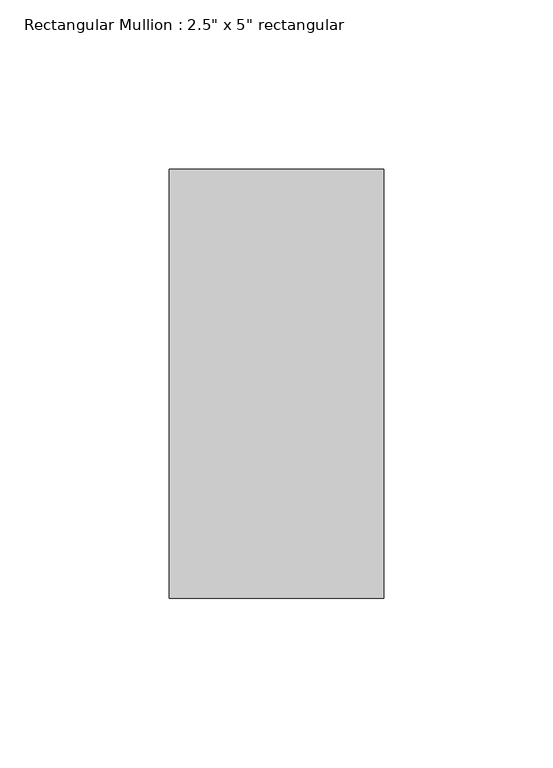
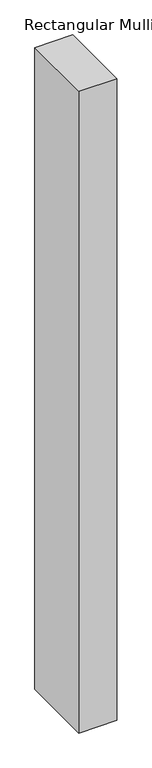
"""IFC4 building model written with IfcOpenShell, lengths in millimetres: member geometry."""

from ifc_helpers import new_model, si_unit, frame, origin, place, context, project, spatial, polyline, outline, extrude, source, transform, mapped, element, save


def member_e3a8255e(model_context):
    return source(origin(), model_context, "Body", "SweptSolid", [
        extrude(outline(polyline([(31.75, 63.5), (31.75, -63.5), (-31.75, -63.5), (-31.75, 63.5), (31.75, 63.5)])), frame((0.0, 0.0, -1132.4166667), z_axis=(0.0, 0.0, 1.0), x_axis=(1.0, 0.0, 0.0)), (0.0, 0.0, 1.0), 1132.4166667),
    ])


if __name__ == "__main__":
    model = new_model("IFC4")
    model_context = context("Model", 3, world=origin())
    ifc_project = project(units=[si_unit("LENGTHUNIT", "METRE", prefix="MILLI")], contexts=[model_context])
    site = spatial("IfcSite", under=ifc_project)
    building = spatial("IfcBuilding", under=site)
    placement = place(None, origin())
    member_shape = member_e3a8255e(model_context)
    element("IfcMember", 1, ObjectType="Rectangular Mullion : 2.5\" x 5\" rectangular", at=placement, inside=building, context=model_context, shape_type="MappedRepresentation", body=[
        mapped(member_shape, transform((0.0, 0.0, 0.0), x_axis=(1.0, 0.0, 0.0), y_axis=(0.0, 1.0, 0.0), z_axis=(0.0, 0.0, 1.0))),
    ])
    save(model, "model.ifc")

# Revit data of these elements
# Type "Rectangular Mullion : 2.5\" x 5\" rectangular"
#   built-in parameter 1007304 = 0.416667 (stored number, unit not read)
#   built-in parameter 1007301 = 0.104167 (stored number, unit not read)
#   built-in parameter 1007300 = 0.104167 (stored number, unit not read)
# Element 1 (IfcMember, "Rectangular Mullion : 2.5\" x 5\" rectangular")
#   Materials on its faces: "Aluminum"
# Materials
#   "Aluminum": class "Metal", colour RGB 247 247 247, transparency 0, Description = "Aluminum 6061", Cost = 0
